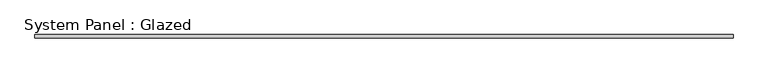
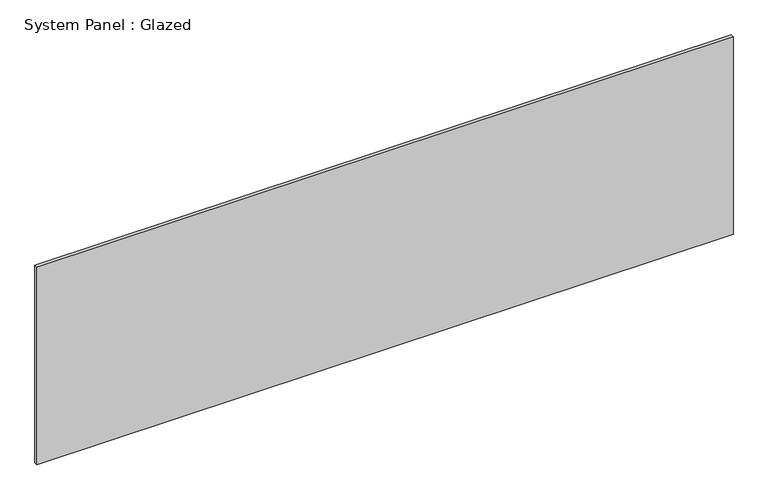
"""IFC4 building model written with IfcOpenShell, lengths in millimetres: plate geometry, System Panel : Glazed."""

from ifc_helpers import new_model, si_unit, origin, origin_with_axes, place, context, project, spatial, polyline, outline, extrude, source, transform, mapped, element, save


def system_panel_glazed_9f3cc7a8(model_context):
    return source(origin(), model_context, "Body", "SweptSolid", [
        extrude(outline(polyline([(2542.0842472, 19.05), (-2542.0842472, 19.05), (-2542.0842472, 44.45), (2542.0842472, 44.45), (2542.0842472, 19.05)])), origin_with_axes(), (0.0, 0.0, 1.0), 1524.0),
    ])


if __name__ == "__main__":
    model = new_model("IFC4")
    model_context = context("Model", 3, world=origin())
    ifc_project = project(units=[si_unit("LENGTHUNIT", "METRE", prefix="MILLI")], contexts=[model_context])
    site = spatial("IfcSite", under=ifc_project)
    building = spatial("IfcBuilding", under=site)
    placement = place(None, origin())
    system_panel_glazed_shape = system_panel_glazed_9f3cc7a8(model_context)
    element("IfcPlate", 1, ObjectType="System Panel : Glazed", at=placement, inside=building, context=model_context, shape_type="MappedRepresentation", body=[
        mapped(system_panel_glazed_shape, transform((0.0, 0.0, 0.0), x_axis=(1.0, 0.0, 0.0), y_axis=(0.0, 1.0, 0.0), z_axis=(0.0, 0.0, 1.0))),
    ])
    save(model, "model.ifc")

# Revit data of these elements
# Type "System Panel : Glazed"
#   Construction Type Id = "GSP4R"
#   Analytic Construction = "1/8 in Pilkington single glazing"
#   Visual Light Transmittance = 0.9
#   Solar Heat Gain Coefficient = 0.86
#   Heat Transfer Coefficient (U) = 1.18115 BTU/(h·ft²·°F)
# Element 1 (IfcPlate, "System Panel : Glazed")
#   Materials on its faces: "Glass"
# Materials
#   "Glass": class "Glass", colour RGB 0 128 192, transparency 0.75, Description = "Soda Lime Glass", Cost = 0
